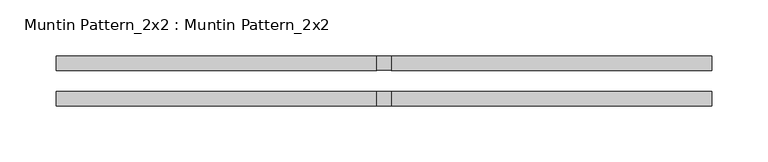
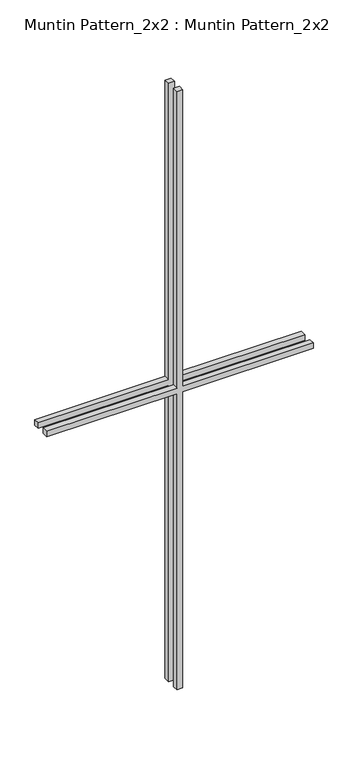
"""IFC4 building model written with IfcOpenShell, lengths in millimetres: proxy geometry, Muntin Pattern_2x2 : Muntin Pattern_2x2."""

from ifc_helpers import new_model, si_unit, frame, origin, place, context, project, spatial, polyline, outline, extrude, source, transform, mapped, element, save


def muntin_pattern_2x2_muntin_pattern_2x2_6849e3ed(model_context):
    return source(origin(), model_context, "Body", "SweptSolid", [
        extrude(outline(polyline([(698.5, -6.35), (698.5, -292.1), (685.8, -292.1), (685.8, -6.35), (0.0, -6.35), (0.0, 6.35), (685.8, 6.35), (685.8, 292.1), (698.5, 292.1), (698.5, 6.35), (1384.3, 6.35), (1384.3, -6.35), (698.5, -6.35)])), frame((0.0, 9.525, 0.0), z_axis=(0.0, 1.0, 0.0), x_axis=(0.0, 0.0, 1.0)), (0.0, 0.0, 1.0), 12.7),
        extrude(outline(polyline([(698.5, -6.35), (698.5, -292.1), (685.8, -292.1), (685.8, -6.35), (0.0, -6.35), (0.0, 6.35), (685.8, 6.35), (685.8, 292.1), (698.5, 292.1), (698.5, 6.35), (1384.3, 6.35), (1384.3, -6.35), (698.5, -6.35)])), frame((0.0, -22.225, 0.0), z_axis=(0.0, 1.0, 0.0), x_axis=(0.0, 0.0, 1.0)), (0.0, 0.0, 1.0), 12.7),
    ])


if __name__ == "__main__":
    model = new_model("IFC4")
    model_context = context("Model", 3, world=origin())
    ifc_project = project(units=[si_unit("LENGTHUNIT", "METRE", prefix="MILLI")], contexts=[model_context])
    site = spatial("IfcSite", under=ifc_project)
    building = spatial("IfcBuilding", under=site)
    placement = place(None, origin())
    muntin_pattern_2x2_muntin_pattern_2x2_shape = muntin_pattern_2x2_muntin_pattern_2x2_6849e3ed(model_context)
    element("IfcBuildingElementProxy", 1, Name="Muntin Pattern_2x2 : Muntin Pattern_2x2", ObjectType="Muntin Pattern_2x2 : Muntin Pattern_2x2", at=placement, inside=building, context=model_context, shape_type="MappedRepresentation", body=[
        mapped(muntin_pattern_2x2_muntin_pattern_2x2_shape, transform((0.0, 0.0, 0.0), x_axis=(1.0, 0.0, 0.0), y_axis=(0.0, 1.0, 0.0), z_axis=(0.0, 0.0, 1.0))),
    ])
    save(model, "model.ifc")

# Revit data of these elements
# Type "Muntin Pattern_2x2 : Muntin Pattern_2x2"
#   Width [instance default] = 4' - 0"
#   Thickness = 0' - 0 1/2"
#   Height [instance default] = 4' - 0"
#   Distance = 0' - 0 3/4"
#   Interior Material [instance default] = none
#   Exterior Material [instance default] = none
#   Default Elevation = 0
# Element 1 (IfcBuildingElementProxy, "Muntin Pattern_2x2 : Muntin Pattern_2x2")
#   Width = 1' - 11"
#   Height = 4' - 6 1/2"
#   Interior Material = Wood - Stained
#   Exterior Material = Clad - White
#   Materials on its faces: "Clad - White", "Wood - Stained"
# Materials
#   "Clad - White": class "Wood", colour RGB 242 242 238, transparency 0, Cost = 0
#   "Wood - Stained": class "Wood", colour RGB 224 178 126, transparency 0, Cost = 0
